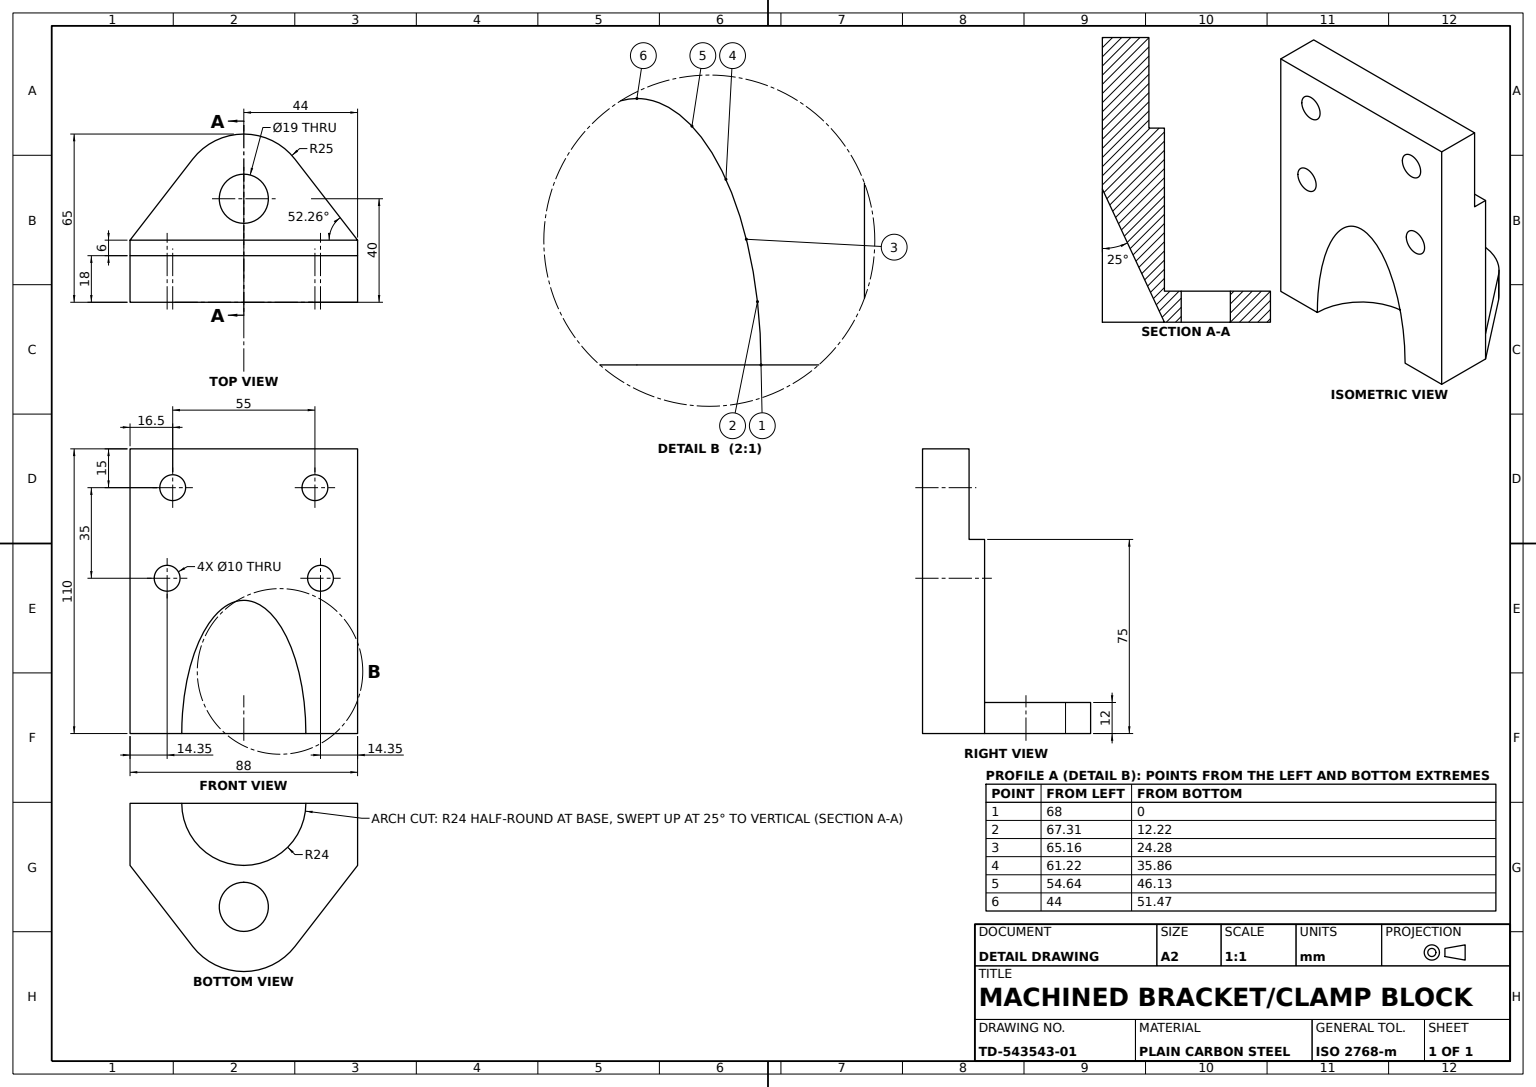
SolidWorks part; units mm, degrees
material "Plain Carbon Steel"
ref_plane "Front Plane" through (0, 0, 0) normal (0, 0, 1) x (1, 0, 0)
ref_plane "Top Plane" through (0, 0, 0) normal (0, 1, 0) x (1, 0, 0)
ref_plane "Right Plane" through (0, 0, 0) normal (1, 0, 0) x (0, 0, -1)
sketch "Base Plate Sketch" plane through (0, 0, 0) normal (0, 0, 1) x (1, 0, 0)
  line L5 (-44, 110) -> (44, 110)
  line L6 (-44, 110) -> (-44, 0)
  line L7 (-44, 0) -> (44, 0)
  line L8 (44, 110) -> (44, 0)
  line L9 (-44, 110) -> (44, 0) construction
  line L10 (-44, 0) -> (44, 110) construction
  point P0 (0, 55)
  dimension "D1" = 88
  dimension "D2" = 110
extrude "Base Plate" add sketch "Base Plate Sketch" against normal blind 18
sketch "Side Boss Sketch" plane through (0, 0, 0) normal (0, 1, 0) x (1, 0, 0)
  line L1 (-44, 24) -> (44, 24)
  line L2 (-44, 24) -> (-44, 18)
  line L3 (-44, 18) -> (44, 18)
  line L4 (44, 24) -> (44, 18)
  line L5 (-44, 24) -> (44, 18) construction
  line L6 (-44, 18) -> (44, 24) construction
  point P0 (0, 21)
  dimension "D1" = 6
  dimension "D2" = 44
extrude "Side Boss" add sketch "Side Boss Sketch" along normal blind 75
sketch "Rear Boss Sketch" plane through (0, 0, 0) normal (0, -1, 0) x (1, 0, 0)
  line L0 (-44, 0) -> (44, 0) construction
  line L1 (-44, -24) -> (-19.7692, -55.3029)
  line L2 (19.7692, -55.3029) -> (44, -24)
  line L7 (44, 0) -> (-44, 0)
  line L8 (-44, 0) -> (-44, -24)
  line L9 (-44, -24) -> (44, -24)
  line L10 (44, -24) -> (44, 0)
  line L11 (44, 0) -> (-44, 0)
  line L12 (-44, 0) -> (-44, -24)
  line L13 (-44, -24) -> (44, -24)
  line L14 (44, -24) -> (44, 0)
  arc A0 (-19.7692, -55.3029) -> (19.7692, -55.3029) centre (0, -40) ccw
  circle A1 centre (0, -40) radius 9.5
  line M11 (-44, -24) -> (44, -24)
  dimension "D1" = 19
  dimension "D2" = 50
  dimension "D3" = 40
  dimension "D4" = 0
extrude "Rear Boss" add sketch "Rear Boss Sketch" against normal blind 12 contours L1 A0 L2 A1 M11
sketch "Angle Reference Sketch 25deg" plane through (0, 0, 0) normal (1, 0, 0) x (0, 0, -1)
  line L0 (24, 0) -> (-15.6176, 84.9602) construction
  line L1 (24, 0) -> (0, 0) construction
  line L2 (0, 0) -> (0, 110) construction
  dimension "D1" = 25
  dimension "D2" = 24
ref_plane "Angled Reference Plane" through (0, 9.1925, -19.7135) normal (0, 0.4226, -0.9063) x (0, 0.9063, 0.4226)
sketch "Angled Cut Sketch" plane through (0, 0, 0) normal (0, 0, 1) x (1, 0, 0)
  line L0 (0, 0) -> (0, 42.4801) construction
  line L1 (0, 0) -> (0, 84.9602) construction
  line L2 (44, 110) -> (-44, 110) construction
  line L3 (44, 0) -> (44, 110) construction
  circle A0 centre (-27.5, 95) radius 5
  circle A1 centre (27.5, 95) radius 5
  circle A2 centre (29.6529, 60) radius 5
  circle A3 centre (-29.6529, 60) radius 5
  dimension "D7" = 10
  dimension "D1" = 35
  dimension "D2" = 116.299
  dimension "D3" = 55
  dimension "D4" = 59.3058
  dimension "D5" = 55
  dimension "D6" = 15
  dimension "D8" = 14.3471
extrude "Angled Cut" cut sketch "Angled Cut Sketch" against normal up to surface (24 mm away) up to face at (0, 43.5, -24)
sketch "Arch Cut Sketch" plane through (0, 0, 0) normal (0, -1, 0) x (1, 0, 0)
  circle A1 centre (0, 0) radius 24
  dimension "D1" = 48
extrude "Arch Cut" cut sketch "Arch Cut Sketch" along direction (0, 0.9063, 0.4226) on the side against the normal up to vertex (84.9602 mm away)
